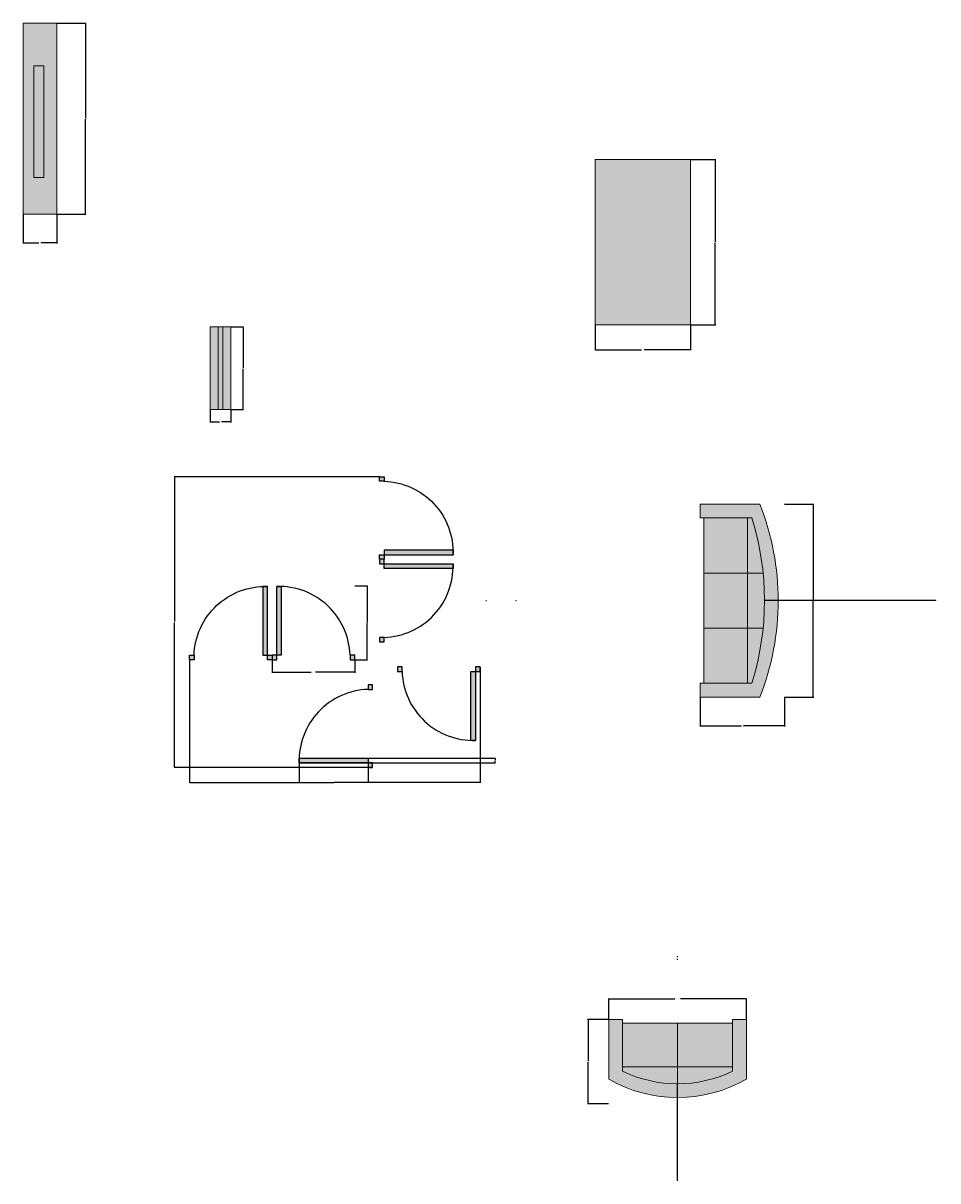
# Model space of a CAD drawing. Units: inches. Extents: x -494 to 1275, y 12 to 1194.
# Tile 5 of 8: x 857 to 1255, y 231 to 735. Entities that reach past the tile are written whole.
import ezdxf

# ---------------------------------------------------------------- set-up
doc = ezdxf.new("R2010")
doc.units = ezdxf.units.IN
doc.header["$MEASUREMENT"] = 0
for name, color, linetype, lineweight in [('A-ANNO-DIMS', 2, 'Continuous', 18), ('A-DOOR', 3, 'Continuous', 25), ('A-DOOR-PATT', 7, 'Continuous', 13), ('A-FURN', 8, 'Continuous', 18), ('A-GLAZ', 4, 'Continuous', 18), ('A-GLAZ-FRAM-PATT', 7, 'Continuous', 13), ('A-GLAZ-GLAS-PATT', 4, 'Continuous', 13)]:
    doc.layers.add(name, color=color, linetype=linetype, lineweight=lineweight)
doc.layers.add('A-FURN-PATT', color=254, linetype='Continuous', lineweight=13, true_color=0xfeeab9)
doc.styles.get("Standard").update_dxf_attribs({"font": 'arial.ttf'})
doc.dimstyles.get("Standard").update_dxf_attribs({"dimtxt": 0.18, "dimasz": 0.18, "dimexe": 0.18, "dimexo": 0.0625, "dimgap": 0.09, "dimtad": 0, "dimtih": 1, "dimtoh": 1, "dimdec": 4, "dimzin": 0, "dimdsep": 46, "dimlunit": 4, "dimtxsty": 'Standard', "dimcen": 0.09, "dimadec": 0, "dimazin": 0, "dimtfac": 1, "dimtdec": 4, "dimtofl": 0, "dimtmove": 0, "dimatfit": 3, "dimfxl": 1, "dimtolj": 1, "dimtzin": 0, "dimarcsym": 0})

# ---------------------------------------------------------------- blocks, each defined once
blk = doc.blocks.new('Sofa - Roundback Loveseat 5 ft.')
for p, q in [((0, -32.44198), (0, -5.99998)), ((-24, -33.99998), (-24, -11.46958)), ((-23.9998, -13.38178), (23.99986, -13.38178)), ((24.00004, -33.99998), (24.00004, -11.46958)), ((-24, -32.44198), (24.00004, -32.44198))]:
    blk.add_line(p, q)
for points in [[(-24, -33.99998), (-30, -33.99998), (-30, -7.99998)], [(30.00004, -7.99998), (30.00004, -33.99998), (24.00004, -33.99998)]]:
    blk.add_lwpolyline(points)
for centre, radius, start, end in [((0, -60.24998), 60.24998, 60.13715, 119.8628), ((0, -61.38438), 55.38444, 64.32083, 115.6792)]:
    blk.add_arc(centre, radius, start, end)
blk = doc.blocks.new('WINDOW-36IN')
for p, q in [((3.5, 36), (3.5, 0)), ((5.5, 36), (5.5, 0))]:
    blk.add_line(p, q)
blk.add_lwpolyline([(0, 36), (9, 36), (9, 0), (0, 0)], close=True)
blk = doc.blocks.new('DOOR-SINGLE-36IN')
blk.add_lwpolyline([(34, 2, 0.414214), (2, 32), (4, 32), (4, 2), (2, 2), (2, 32)], format="xyb")
for points in [[(0, 0), (2, 0), (2, 2), (0, 2)], [(34, 0), (36, 0), (36, 2), (34, 2)]]:
    blk.add_lwpolyline(points, close=True)
blk = doc.blocks.new('SOFA-84IN-PLAN')
h = blk.add_hatch(color=256)
h.dxf.hatch_style = 1
h.paths.add_polyline_path([(20.62, 54), (1.56, 54), (1.56, 30), (20.62, 30)], flags=17)
h.paths.add_polyline_path([(20.62, 78), (1.56, 78), (1.56, 54), (20.62, 54)], flags=17)
h.paths.add_polyline_path([(22.53, 78), (20.62, 78), (20.62, 54), (27.4, 54, 0.050647)], flags=17)
h.paths.add_polyline_path([(27.4, 54), (20.62, 54), (20.62, 30), (27.4, 30, 0.049628)], flags=17)
h.paths.add_polyline_path([(20.62, 30), (1.56, 30), (1.56, 6), (20.62, 6)], flags=17)
h.paths.add_polyline_path([(27.4, 30), (20.62, 30), (20.62, 6), (22.53, 6, 0.050647)], flags=17)
h.paths.add_polyline_path([(26, 84), (0, 84), (0, 78), (22.53, 78, -0.050647), (27.4, 54, -0.100528), (22.53, 6), (20.62, 6), (1.56, 6), (0, 6), (0, 0), (26, 0, 0.190476)])
for p, q in [((0, 78), (22.53, 78)), ((1.56, 78), (1.56, 6)), ((20.62, 78), (20.62, 6)), ((1.56, 54), (27.4, 54)), ((1.56, 30), (27.4, 30)), ((0, 6), (22.53, 6))]:
    blk.add_line(p, q)
for points in [[(0, 78), (0, 84), (26, 84)], [(26, 0), (0, 0), (0, 6)]]:
    blk.add_lwpolyline(points)
for centre, radius, start, end in [((-80.25, 42), 114.25, 338.4314, 21.5686), ((-93.2, 42), 121.2, 342.7203, 17.2797)]:
    blk.add_arc(centre, radius, start, end)
blk = doc.blocks.new('TABLE-RECTANGULAR-72IN')
h = blk.add_hatch(color=256)
h.dxf.hatch_style = 1
h.paths.add_polyline_path([(41.56, 71.99), (0, 71.99), (0, 0), (41.56, 0)])
blk.add_lwpolyline([(0, 0), (41.56, 0), (41.56, 71.99), (0, 71.99)], close=True)
blk = doc.blocks.new('MEDIA-CONSOLE-PLAN')
for p, q in [((4.67, 64.59), (9.03, 64.59)), ((4.67, 16.07), (4.67, 64.59)), ((9.03, 64.59), (9.03, 16.07)), ((9.03, 16.07), (4.67, 16.07))]:
    blk.add_line(p, q)
blk.add_lwpolyline([(0, 83.25), (14.68, 83.25), (14.68, 0), (0, 0)], close=True)
blk = doc.blocks.new('*D18')
at = {"layer": 'A-ANNO-DIMS', "color": 0, "lineweight": -2, "transparency": 16777216}
for p, q in [((965.19, 457.67), (965.19, 452.15)), ((1001.19, 457.67), (1001.19, 452.15)), ((965.37, 452.33), (982.25, 452.33)), ((1001.01, 452.33), (984.12, 452.33))]:
    blk.add_line(p, q, dxfattribs=at)
at = {"layer": 'A-ANNO-DIMS', "color": 0, "transparency": 16777216}
for points in [[(965.37, 452.36), (965.37, 452.3), (965.19, 452.33)], [(1001.01, 452.36), (1001.01, 452.3), (1001.19, 452.33)]]:
    blk.add_solid(points, dxfattribs=at)
at = {"layer": 'Defpoints', "color": 0, "transparency": 16777216}
for p in [(965.19, 457.73), (1001.19, 457.73), (1001.19, 452.33)]:
    blk.add_point(p, dxfattribs=at)
at = {"layer": 'A-ANNO-DIMS', "color": 0, "transparency": 16777216, "insert": (983.19, 452.33), "char_height": 0.18, "attachment_point": 5}
blk.add_mtext('\\A1;DOOR 36 TYP.', dxfattribs=at)
blk = doc.blocks.new('*D19')
at = {"layer": 'A-ANNO-DIMS', "color": 0, "lineweight": -2, "transparency": 16777216}
for p, q in [((1001.25, 490), (1006.77, 490)), ((1006.59, 489.82), (1006.59, 474.05)), ((1006.59, 457.91), (1006.59, 473.68)), ((1001.25, 457.73), (1006.77, 457.73))]:
    blk.add_line(p, q, dxfattribs=at)
at = {"layer": 'A-ANNO-DIMS', "color": 0, "transparency": 16777216}
for points in [[(1006.56, 489.82), (1006.62, 489.82), (1006.59, 490)], [(1006.56, 457.91), (1006.62, 457.91), (1006.59, 457.73)]]:
    blk.add_solid(points, dxfattribs=at)
at = {"layer": 'Defpoints', "color": 0, "transparency": 16777216}
for p in [(1001.19, 490), (1006.59, 490), (1001.19, 457.73)]:
    blk.add_point(p, dxfattribs=at)
at = {"layer": 'A-ANNO-DIMS', "color": 0, "transparency": 16777216, "insert": (1006.59, 473.86), "char_height": 0.18, "attachment_point": 5}
blk.add_mtext('\\A1;32 TYP.', dxfattribs=at)
blk = doc.blocks.new('*D22')
at = {"layer": 'A-ANNO-DIMS', "color": 0, "lineweight": -2, "transparency": 16777216}
for p, q in [((947.28, 602.76), (952.8, 602.76)), ((952.62, 602.58), (952.62, 584.95)), ((952.62, 566.94), (952.62, 584.58)), ((947.28, 566.76), (952.8, 566.76))]:
    blk.add_line(p, q, dxfattribs=at)
at = {"layer": 'A-ANNO-DIMS', "color": 0, "transparency": 16777216}
for points in [[(952.59, 602.58), (952.65, 602.58), (952.62, 602.76)], [(952.59, 566.94), (952.65, 566.94), (952.62, 566.76)]]:
    blk.add_solid(points, dxfattribs=at)
at = {"layer": 'Defpoints', "color": 0, "transparency": 16777216}
for p in [(947.22, 602.76), (952.62, 602.76), (947.22, 566.76)]:
    blk.add_point(p, dxfattribs=at)
at = {"layer": 'A-ANNO-DIMS', "color": 0, "transparency": 16777216, "insert": (952.62, 584.76), "char_height": 0.18, "attachment_point": 5}
blk.add_mtext('\\A1;WINDOW B 36 TYP.', dxfattribs=at)
blk = doc.blocks.new('*D23')
at = {"layer": 'A-ANNO-DIMS', "color": 0, "lineweight": -2, "transparency": 16777216}
for p, q in [((938.22, 566.7), (938.22, 561.18)), ((947.22, 566.7), (947.22, 561.18)), ((938.4, 561.36), (942.26, 561.36)), ((947.04, 561.36), (943.18, 561.36))]:
    blk.add_line(p, q, dxfattribs=at)
at = {"layer": 'A-ANNO-DIMS', "color": 0, "transparency": 16777216}
for points in [[(938.4, 561.39), (938.4, 561.33), (938.22, 561.36)], [(947.04, 561.39), (947.04, 561.33), (947.22, 561.36)]]:
    blk.add_solid(points, dxfattribs=at)
at = {"layer": 'Defpoints', "color": 0, "transparency": 16777216}
for p in [(938.22, 566.76), (947.22, 566.76), (947.22, 561.36)]:
    blk.add_point(p, dxfattribs=at)
at = {"layer": 'A-ANNO-DIMS', "color": 0, "transparency": 16777216, "insert": (942.72, 561.36), "char_height": 0.18, "attachment_point": 5}
blk.add_mtext('\\A1;9 TYP.', dxfattribs=at)
blk = doc.blocks.new('*D28')
at = {"layer": 'A-ANNO-DIMS', "color": 0, "lineweight": -2, "transparency": 16777216}
for p, q in [((1111.85, 301.15), (1111.85, 310.27)), ((1112.03, 310.09), (1140.63, 310.09)), ((1171.67, 310.09), (1143.08, 310.09)), ((1171.85, 301.15), (1171.85, 310.27))]:
    blk.add_line(p, q, dxfattribs=at)
at = {"layer": 'A-ANNO-DIMS', "color": 0, "transparency": 16777216}
for points in [[(1112.03, 310.12), (1112.03, 310.06), (1111.85, 310.09)], [(1171.67, 310.12), (1171.67, 310.06), (1171.85, 310.09)]]:
    blk.add_solid(points, dxfattribs=at)
at = {"layer": 'Defpoints', "color": 0, "transparency": 16777216}
for p in [(1111.85, 310.09), (1111.85, 301.09), (1171.85, 301.09)]:
    blk.add_point(p, dxfattribs=at)
at = {"layer": 'A-ANNO-DIMS', "color": 0, "transparency": 16777216, "insert": (1141.85, 310.09), "char_height": 0.18, "attachment_point": 5}
blk.add_mtext('\\A1;LOVESEAT 60 TYP.', dxfattribs=at)
blk = doc.blocks.new('*D29')
at = {"layer": 'A-ANNO-DIMS', "color": 0, "lineweight": -2, "transparency": 16777216}
for p, q in [((1111.79, 301.09), (1102.67, 301.09)), ((1102.85, 300.91), (1102.85, 282.94)), ((1102.85, 264.6), (1102.85, 282.57)), ((1111.79, 264.42), (1102.67, 264.42))]:
    blk.add_line(p, q, dxfattribs=at)
at = {"layer": 'A-ANNO-DIMS', "color": 0, "transparency": 16777216}
for points in [[(1102.82, 300.91), (1102.88, 300.91), (1102.85, 301.09)], [(1102.82, 264.6), (1102.88, 264.6), (1102.85, 264.42)]]:
    blk.add_solid(points, dxfattribs=at)
at = {"layer": 'Defpoints', "color": 0, "transparency": 16777216}
for p in [(1111.85, 301.09), (1102.85, 264.42), (1111.85, 264.42)]:
    blk.add_point(p, dxfattribs=at)
at = {"layer": 'A-ANNO-DIMS', "color": 0, "transparency": 16777216, "insert": (1102.85, 282.76), "char_height": 0.18, "attachment_point": 5}
blk.add_mtext('\\A1;37 TYP.', dxfattribs=at)
blk = doc.blocks.new('*D32')
at = {"layer": 'A-ANNO-DIMS', "color": 0, "lineweight": -2, "transparency": 16777216}
for p, q in [((1188.46, 525.54), (1201.18, 525.54)), ((1201, 525.36), (1201, 483.73)), ((1201, 441.72), (1201, 483.36)), ((1188.46, 441.54), (1201.18, 441.54))]:
    blk.add_line(p, q, dxfattribs=at)
at = {"layer": 'A-ANNO-DIMS', "color": 0, "transparency": 16777216}
for points in [[(1200.97, 525.36), (1201.03, 525.36), (1201, 525.54)], [(1200.97, 441.72), (1201.03, 441.72), (1201, 441.54)]]:
    blk.add_solid(points, dxfattribs=at)
at = {"layer": 'Defpoints', "color": 0, "transparency": 16777216}
for p in [(1188.4, 525.54), (1201, 525.54), (1188.4, 441.54)]:
    blk.add_point(p, dxfattribs=at)
at = {"layer": 'A-ANNO-DIMS', "color": 0, "transparency": 16777216, "insert": (1201, 483.54), "char_height": 0.18, "attachment_point": 5}
blk.add_mtext('\\A1;SOFA 84 TYP.', dxfattribs=at)
blk = doc.blocks.new('*D33')
at = {"layer": 'A-ANNO-DIMS', "color": 0, "lineweight": -2, "transparency": 16777216}
for p, q in [((1151.73, 441.48), (1151.73, 428.76)), ((1188.4, 441.48), (1188.4, 428.76)), ((1151.91, 428.94), (1169.53, 428.94)), ((1188.22, 428.94), (1170.59, 428.94))]:
    blk.add_line(p, q, dxfattribs=at)
at = {"layer": 'A-ANNO-DIMS', "color": 0, "transparency": 16777216}
for points in [[(1151.91, 428.97), (1151.91, 428.91), (1151.73, 428.94)], [(1188.22, 428.97), (1188.22, 428.91), (1188.4, 428.94)]]:
    blk.add_solid(points, dxfattribs=at)
at = {"layer": 'Defpoints', "color": 0, "transparency": 16777216}
for p in [(1151.73, 441.54), (1188.4, 441.54), (1188.4, 428.94)]:
    blk.add_point(p, dxfattribs=at)
at = {"layer": 'A-ANNO-DIMS', "color": 0, "transparency": 16777216, "insert": (1170.06, 428.94), "char_height": 0.18, "attachment_point": 5}
blk.add_mtext('\\A1;37 TYP.', dxfattribs=at)
blk = doc.blocks.new('*D34')
at = {"layer": 'A-ANNO-DIMS', "color": 0, "lineweight": -2, "transparency": 16777216}
for p, q in [((1147.57, 675.62), (1158.48, 675.62)), ((1158.3, 675.44), (1158.3, 639.81)), ((1158.3, 603.81), (1158.3, 639.44)), ((1147.57, 603.63), (1158.48, 603.63))]:
    blk.add_line(p, q, dxfattribs=at)
at = {"layer": 'A-ANNO-DIMS', "color": 0, "transparency": 16777216}
for points in [[(1158.27, 675.44), (1158.33, 675.44), (1158.3, 675.62)], [(1158.27, 603.81), (1158.33, 603.81), (1158.3, 603.63)]]:
    blk.add_solid(points, dxfattribs=at)
at = {"layer": 'Defpoints', "color": 0, "transparency": 16777216}
for p in [(1147.5, 675.62), (1158.3, 675.62), (1147.5, 603.63)]:
    blk.add_point(p, dxfattribs=at)
at = {"layer": 'A-ANNO-DIMS', "color": 0, "transparency": 16777216, "insert": (1158.3, 639.63), "char_height": 0.18, "attachment_point": 5}
blk.add_mtext('\\A1;TABLE 72 TYP.', dxfattribs=at)
blk = doc.blocks.new('*D35')
at = {"layer": 'A-ANNO-DIMS', "color": 0, "lineweight": -2, "transparency": 16777216}
for p, q in [((1105.94, 603.57), (1105.94, 592.65)), ((1147.5, 603.57), (1147.5, 592.65)), ((1106.12, 592.83), (1126.19, 592.83)), ((1147.32, 592.83), (1127.25, 592.83))]:
    blk.add_line(p, q, dxfattribs=at)
at = {"layer": 'A-ANNO-DIMS', "color": 0, "transparency": 16777216}
for points in [[(1106.12, 592.86), (1106.12, 592.8), (1105.94, 592.83)], [(1147.32, 592.86), (1147.32, 592.8), (1147.5, 592.83)]]:
    blk.add_solid(points, dxfattribs=at)
at = {"layer": 'Defpoints', "color": 0, "transparency": 16777216}
for p in [(1105.94, 603.63), (1147.5, 603.63), (1147.5, 592.83)]:
    blk.add_point(p, dxfattribs=at)
at = {"layer": 'A-ANNO-DIMS', "color": 0, "transparency": 16777216, "insert": (1126.72, 592.83), "char_height": 0.18, "attachment_point": 5}
blk.add_mtext('\\A1;42 TYP.', dxfattribs=at)
blk = doc.blocks.new('*D36')
at = {"layer": 'A-ANNO-DIMS', "color": 0, "lineweight": -2, "transparency": 16777216}
for p, q in [((871.45, 735.08), (884.06, 735.08)), ((883.88, 734.9), (883.88, 693.64)), ((883.88, 652.01), (883.88, 693.27)), ((871.45, 651.83), (884.06, 651.83))]:
    blk.add_line(p, q, dxfattribs=at)
at = {"layer": 'A-ANNO-DIMS', "color": 0, "transparency": 16777216}
for points in [[(883.85, 734.9), (883.91, 734.9), (883.88, 735.08)], [(883.85, 652.01), (883.91, 652.01), (883.88, 651.83)]]:
    blk.add_solid(points, dxfattribs=at)
at = {"layer": 'Defpoints', "color": 0, "transparency": 16777216}
for p in [(871.39, 735.08), (883.88, 735.08), (871.39, 651.83)]:
    blk.add_point(p, dxfattribs=at)
at = {"layer": 'A-ANNO-DIMS', "color": 0, "transparency": 16777216, "insert": (883.88, 693.45), "char_height": 0.18, "attachment_point": 5}
blk.add_mtext('\\A1;CONSOLE 83 TYP.', dxfattribs=at)
blk = doc.blocks.new('*D37')
at = {"layer": 'A-ANNO-DIMS', "color": 0, "lineweight": -2, "transparency": 16777216}
for p, q in [((856.71, 651.77), (856.71, 639.16)), ((871.39, 651.77), (871.39, 639.16)), ((856.89, 639.34), (863.53, 639.34)), ((871.21, 639.34), (864.57, 639.34))]:
    blk.add_line(p, q, dxfattribs=at)
at = {"layer": 'A-ANNO-DIMS', "color": 0, "transparency": 16777216}
for points in [[(856.89, 639.37), (856.89, 639.31), (856.71, 639.34)], [(871.21, 639.37), (871.21, 639.31), (871.39, 639.34)]]:
    blk.add_solid(points, dxfattribs=at)
at = {"layer": 'Defpoints', "color": 0, "transparency": 16777216}
for p in [(856.71, 651.83), (871.39, 651.83), (871.39, 639.34)]:
    blk.add_point(p, dxfattribs=at)
at = {"layer": 'A-ANNO-DIMS', "color": 0, "transparency": 16777216, "insert": (864.05, 639.34), "char_height": 0.18, "attachment_point": 5}
blk.add_mtext('\\A1;15 TYP.', dxfattribs=at)
blk = doc.blocks.new('*D76')
at = {"layer": 'A-ANNO-DIMS', "color": 0, "lineweight": -2, "transparency": 16777216}
for p, q in [((929.19, 457.67), (929.19, 404.15)), ((1055.84, 454.62), (1055.84, 404.15)), ((929.37, 404.33), (992.06, 404.33)), ((1055.66, 404.33), (992.97, 404.33))]:
    blk.add_line(p, q, dxfattribs=at)
at = {"layer": 'A-ANNO-DIMS', "color": 0, "transparency": 16777216}
for points in [[(929.37, 404.36), (929.37, 404.3), (929.19, 404.33)], [(1055.66, 404.36), (1055.66, 404.3), (1055.84, 404.33)]]:
    blk.add_solid(points, dxfattribs=at)
at = {"layer": 'Defpoints', "color": 0, "transparency": 16777216}
for p in [(929.19, 457.73), (1055.84, 454.69), (1055.84, 404.33)]:
    blk.add_point(p, dxfattribs=at)
at = {"layer": 'A-ANNO-DIMS', "color": 0, "transparency": 16777216, "insert": (992.51, 404.33), "char_height": 0.18, "attachment_point": 5}
blk.add_mtext('\\A1;126.66', dxfattribs=at)
blk = doc.blocks.new('*D77')
at = {"layer": 'A-ANNO-DIMS', "color": 0, "lineweight": -2, "transparency": 16777216}
for p, q in [((1011.97, 537.54), (922.46, 537.54)), ((922.64, 537.36), (922.64, 474.39)), ((922.64, 411.06), (922.64, 474.03)), ((1008.93, 410.88), (922.46, 410.88))]:
    blk.add_line(p, q, dxfattribs=at)
at = {"layer": 'A-ANNO-DIMS', "color": 0, "transparency": 16777216}
for points in [[(922.61, 537.36), (922.67, 537.36), (922.64, 537.54)], [(922.61, 411.06), (922.67, 411.06), (922.64, 410.88)]]:
    blk.add_solid(points, dxfattribs=at)
at = {"layer": 'Defpoints', "color": 0, "transparency": 16777216}
for p in [(922.64, 537.54), (1012.04, 537.54), (1008.99, 410.88)]:
    blk.add_point(p, dxfattribs=at)
at = {"layer": 'A-ANNO-DIMS', "color": 0, "transparency": 16777216, "insert": (922.64, 474.21), "char_height": 0.18, "attachment_point": 5}
blk.add_mtext('\\A1;126.66', dxfattribs=at)
blk = doc.blocks.new('*D95')
at = {"layer": 'A-ANNO-DIMS', "color": 0, "lineweight": -2, "transparency": 16777216}
for p, q in [((976.99, 412.82), (976.99, 404.15)), ((1006.99, 412.82), (1006.99, 404.15)), ((977.17, 404.33), (991.77, 404.33)), ((1006.81, 404.33), (992.21, 404.33))]:
    blk.add_line(p, q, dxfattribs=at)
at = {"layer": 'A-ANNO-DIMS', "color": 0, "transparency": 16777216}
for points in [[(977.17, 404.36), (977.17, 404.3), (976.99, 404.33)], [(1006.81, 404.36), (1006.81, 404.3), (1006.99, 404.33)]]:
    blk.add_solid(points, dxfattribs=at)
at = {"layer": 'Defpoints', "color": 0, "transparency": 16777216}
for p in [(976.99, 412.88), (1006.99, 412.88), (1006.99, 404.33)]:
    blk.add_point(p, dxfattribs=at)
at = {"layer": 'A-ANNO-DIMS', "color": 0, "transparency": 16777216, "insert": (991.99, 404.33), "char_height": 0.18, "attachment_point": 5}
blk.add_mtext('\\A1;30', dxfattribs=at)
blk = doc.blocks.new('*D96')
at = {"layer": 'A-ANNO-DIMS', "color": 0, "lineweight": -2, "transparency": 16777216}
for p, q in [((977.05, 414.88), (1062.57, 414.88)), ((1062.39, 414.7), (1062.39, 414.06)), ((1062.39, 413.06), (1062.39, 413.7)), ((977.05, 412.88), (1062.57, 412.88))]:
    blk.add_line(p, q, dxfattribs=at)
at = {"layer": 'A-ANNO-DIMS', "color": 0, "transparency": 16777216}
for points in [[(1062.36, 414.7), (1062.42, 414.7), (1062.39, 414.88)], [(1062.36, 413.06), (1062.42, 413.06), (1062.39, 412.88)]]:
    blk.add_solid(points, dxfattribs=at)
at = {"layer": 'Defpoints', "color": 0, "transparency": 16777216}
for p in [(976.99, 414.88), (1062.39, 414.88), (976.99, 412.88)]:
    blk.add_point(p, dxfattribs=at)
at = {"layer": 'A-ANNO-DIMS', "color": 0, "transparency": 16777216, "insert": (1062.39, 413.88), "char_height": 0.18, "attachment_point": 5}
blk.add_mtext('\\A1;2', dxfattribs=at)
blk = doc.blocks.new('*D109')
at = {"layer": 'A-ANNO-DIMS', "color": 0, "lineweight": -2, "transparency": 16777216}
for p, q in [((1071.39, 483.54), (1071.57, 483.54)), ((1071.48, 483.45), (1071.48, 483.63)), ((1254.28, 483.54), (1185.91, 483.54))]:
    blk.add_line(p, q, dxfattribs=at)
at = {"layer": 'A-ANNO-DIMS', "color": 0, "transparency": 16777216}
blk.add_solid([(1185.91, 483.57), (1185.91, 483.51), (1185.73, 483.54)], dxfattribs=at)
at = {"layer": 'Defpoints', "color": 0, "transparency": 16777216}
for p in [(1071.48, 483.54), (1185.73, 483.54)]:
    blk.add_point(p, dxfattribs=at)
at = {"layer": 'A-ANNO-DIMS', "color": 0, "transparency": 16777216, "insert": (1254.83, 483.54), "char_height": 0.18, "attachment_point": 5}
blk.add_mtext('\\A1;R114.25', dxfattribs=at)
blk = doc.blocks.new('*D110')
at = {"layer": 'A-ANNO-DIMS', "color": 0, "lineweight": -2, "transparency": 16777216}
for p, q in [((1058.44, 483.54), (1058.62, 483.54)), ((1058.53, 483.45), (1058.53, 483.63)), ((1252.45, 483.54), (1179.91, 483.54))]:
    blk.add_line(p, q, dxfattribs=at)
at = {"layer": 'A-ANNO-DIMS', "color": 0, "transparency": 16777216}
blk.add_solid([(1179.91, 483.57), (1179.91, 483.51), (1179.73, 483.54)], dxfattribs=at)
at = {"layer": 'Defpoints', "color": 0, "transparency": 16777216}
for p in [(1058.53, 483.54), (1179.73, 483.54)]:
    blk.add_point(p, dxfattribs=at)
at = {"layer": 'A-ANNO-DIMS', "color": 0, "transparency": 16777216, "insert": (1252.93, 483.54), "char_height": 0.18, "attachment_point": 5}
blk.add_mtext('\\A1;R121.2', dxfattribs=at)
blk = doc.blocks.new('*D111')
at = {"layer": 'A-ANNO-DIMS', "color": 0, "lineweight": -2, "transparency": 16777216}
for p, q in [((1141.76, 327.34), (1141.94, 327.34)), ((1141.85, 327.25), (1141.85, 327.43)), ((1141.85, 230.94), (1141.85, 266.91)), ((1142.04, 230.94), (1141.85, 230.94))]:
    blk.add_line(p, q, dxfattribs=at)
at = {"layer": 'A-ANNO-DIMS', "color": 0, "transparency": 16777216}
blk.add_solid([(1141.89, 266.91), (1141.83, 266.91), (1141.85, 267.09)], dxfattribs=at)
at = {"layer": 'Defpoints', "color": 0, "transparency": 16777216}
for p in [(1141.85, 327.34), (1141.85, 267.09)]:
    blk.add_point(p, dxfattribs=at)
at = {"layer": 'A-ANNO-DIMS', "color": 0, "transparency": 16777216, "insert": (1142.52, 230.94), "char_height": 0.18, "attachment_point": 5}
blk.add_mtext('\\A1;R60.25', dxfattribs=at)
blk = doc.blocks.new('*D112')
at = {"layer": 'A-ANNO-DIMS', "color": 0, "lineweight": -2, "transparency": 16777216}
for p, q in [((1141.76, 328.47), (1141.94, 328.47)), ((1141.85, 328.38), (1141.85, 328.56)), ((1141.85, 239.86), (1141.85, 272.91)), ((1142.04, 239.86), (1141.85, 239.86))]:
    blk.add_line(p, q, dxfattribs=at)
at = {"layer": 'A-ANNO-DIMS', "color": 0, "transparency": 16777216}
blk.add_solid([(1141.89, 272.91), (1141.83, 272.91), (1141.85, 273.09)], dxfattribs=at)
at = {"layer": 'Defpoints', "color": 0, "transparency": 16777216}
for p in [(1141.85, 328.47), (1141.85, 273.09)]:
    blk.add_point(p, dxfattribs=at)
at = {"layer": 'A-ANNO-DIMS', "color": 0, "transparency": 16777216, "insert": (1142.52, 239.86), "char_height": 0.18, "attachment_point": 5}
blk.add_mtext('\\A1;R55.38', dxfattribs=at)

msp = doc.modelspace()

# ---------------------------------------------------------------- hatches: boundary and pattern name
at = {"layer": 'A-DOOR-PATT'}
h = msp.add_hatch(color=256, dxfattribs=at)
h.dxf.hatch_style = 1
h.paths.add_polyline_path([(1044.0365, 503.5367), (1044.0365, 505.5367), (1014.0365, 505.5367), (1014.0365, 503.5367)])
h.paths.add_polyline_path([(1012.0365, 501.5367), (1014.0365, 501.5367), (1014.0365, 503.5367), (1012.0365, 503.5367)])
h.paths.add_polyline_path([(1014.0365, 535.5367), (1014.0365, 537.5367), (1012.0365, 537.5367), (1012.0365, 535.5367)])
h = msp.add_hatch(color=256, dxfattribs=at)
h.dxf.hatch_style = 1
h.paths.add_polyline_path([(1014.0365, 499.5367), (1014.0365, 497.5367), (1044.0365, 497.5367), (1044.0365, 499.5367)])
h.paths.add_polyline_path([(1012.0365, 499.5367), (1014.0365, 499.5367), (1014.0365, 501.5367), (1012.0365, 501.5367)])
h.paths.add_polyline_path([(1012.0365, 467.5367), (1012.0365, 465.5367), (1014.0365, 465.5367), (1014.0365, 467.5367)])
h = msp.add_hatch(color=256, dxfattribs=at)
h.dxf.hatch_style = 1
h.paths.add_polyline_path([(963.1857, 489.7319), (961.1857, 489.7319), (961.1857, 459.7319), (963.1857, 459.7319)])
h.paths.add_polyline_path([(965.1857, 457.7319), (965.1857, 459.7319), (963.1857, 459.7319), (963.1857, 457.7319)])
h.paths.add_polyline_path([(931.1857, 459.7319), (929.1857, 459.7319), (929.1857, 457.7319), (931.1857, 457.7319)])
h = msp.add_hatch(color=256, dxfattribs=at)
h.dxf.hatch_style = 1
h.paths.add_polyline_path([(967.1857, 459.7319), (969.1857, 459.7319), (969.1857, 489.7319), (967.1857, 489.7319)])
h.paths.add_polyline_path([(967.1857, 457.7319), (967.1857, 459.7319), (965.1857, 459.7319), (965.1857, 457.7319)])
h.paths.add_polyline_path([(999.1857, 457.7319), (1001.1857, 457.7319), (1001.1857, 459.7319), (999.1857, 459.7319)])
h = msp.add_hatch(color=256, dxfattribs=at)
h.dxf.hatch_style = 1
h.paths.add_polyline_path([(1053.8413, 452.6859), (1051.8413, 452.6859), (1051.8413, 422.6859), (1053.8413, 422.6859)])
h.paths.add_polyline_path([(1053.8413, 454.6859), (1053.8413, 452.6859), (1055.8413, 452.6859), (1055.8413, 454.6859)])
h.paths.add_polyline_path([(1021.8413, 454.6859), (1019.8413, 454.6859), (1019.8413, 452.6859), (1021.8413, 452.6859)])
h = msp.add_hatch(color=256, dxfattribs=at)
h.dxf.hatch_style = 1
h.paths.add_polyline_path([(1006.9905, 412.8811), (1006.9905, 414.8811), (976.9905, 414.8811), (976.9905, 412.8811)])
h.paths.add_polyline_path([(1008.9905, 412.8811), (1006.9905, 412.8811), (1006.9905, 410.8811), (1008.9905, 410.8811)])
h.paths.add_polyline_path([(1008.9905, 444.8811), (1008.9905, 446.8811), (1006.9905, 446.8811), (1006.9905, 444.8811)])
at = {"layer": 'A-FURN-PATT'}
h = msp.add_hatch(color=256, dxfattribs=at)
h.dxf.hatch_style = 1
h.paths.add_polyline_path([(856.7136, 651.8301), (871.3923, 651.8301), (871.3923, 735.0769), (856.7136, 735.0769)])
h.paths.add_polyline_path([(861.3852, 667.9018), (861.3852, 716.4203), (865.7447, 716.4203), (865.7447, 667.9018)], flags=16)
h = msp.add_hatch(color=256, dxfattribs=at)
h.dxf.hatch_style = 1
h.paths.add_polyline_path([(865.7447, 716.4203), (861.3852, 716.4203), (861.3852, 667.9018), (865.7447, 667.9018)])
h = msp.add_hatch(color=256, dxfattribs=at)
h.dxf.hatch_style = 1
h.paths.add_polyline_path([(1165.8549, 299.5316), (1141.8549, 299.5316), (1141.8549, 280.4714), (1165.8549, 280.4714)], flags=17)
h.paths.add_polyline_path([(1117.8549, 299.5316), (1117.8549, 280.4714), (1141.8549, 280.4714), (1141.8549, 299.5316)], flags=17)
h.paths.add_polyline_path([(1141.8549, 273.0896), (1141.8549, 280.4714), (1117.8549, 280.4714), (1117.8549, 278.5598, 0.11251889)], flags=16)
h.paths.add_polyline_path([(1165.8549, 278.5597), (1165.8549, 280.4714), (1141.8549, 280.4714), (1141.8549, 273.0896, 0.11251869)], flags=17)
h.paths.add_polyline_path([(1117.8549, 278.5598), (1117.8549, 301.0896), (1111.8549, 301.0896), (1111.8549, 275.0897, 0.26666697), (1171.8549, 275.0896), (1171.8549, 301.0896), (1165.8549, 301.0896), (1165.8549, 278.5597, -0.22792319)])
at = {"layer": 'A-GLAZ-FRAM-PATT'}
h = msp.add_hatch(color=256, dxfattribs=at)
h.dxf.hatch_style = 1
h.paths.add_polyline_path([(941.7213, 602.762), (938.2213, 602.762), (938.2213, 566.762), (941.7213, 566.762)])
h.paths.add_polyline_path([(943.7213, 566.762), (947.2213, 566.762), (947.2213, 602.762), (943.7213, 602.762)])
at = {"layer": 'A-GLAZ-GLAS-PATT'}
h = msp.add_hatch(color=256, dxfattribs=at)
h.dxf.hatch_style = 1
h.paths.add_polyline_path([(941.7213, 566.762), (943.7213, 566.762), (943.7213, 602.762), (941.7213, 602.762)])

# ---------------------------------------------------------------- linework, layer by layer
at = {"layer": 'A-DOOR'}
for p, q in [((1012.0365, 535.5367), (1012.0365, 537.5367)), ((1012.0365, 501.5367), (1012.0365, 503.5367)), ((1012.0365, 501.5367), (1012.0365, 499.5367)), ((1012.0365, 467.5367), (1012.0365, 465.5367)), ((931.1857, 457.7319), (929.1857, 457.7319)), ((965.1857, 457.7319), (963.1857, 457.7319)), ((965.1857, 457.7319), (967.1857, 457.7319)), ((999.1857, 457.7319), (1001.1857, 457.7319)), ((1021.8413, 454.6859), (1019.8413, 454.6859)), ((1055.8413, 454.6859), (1053.8413, 454.6859)), ((1008.9905, 444.8811), (1008.9905, 446.8811)), ((1008.9905, 410.8811), (1008.9905, 412.8811))]:
    msp.add_line(p, q, dxfattribs=at)

# ---------------------------------------------------------------- block references
at = {"layer": 'A-DOOR', "extrusion": (0, 0, -1), "zscale": -1, "rotation": 89.99999999999955}
msp.add_blockref('DOOR-SINGLE-36IN', (-1012.0366, 501.537), dxfattribs=at)
at = {"layer": 'A-DOOR'}
for p, rotation in [((1012.0366, 501.5364), 269.9999999999996), ((1055.841, 454.6858), 180), ((1008.9904, 410.8814), 90.0000000000003)]:
    msp.add_blockref('DOOR-SINGLE-36IN', p, dxfattribs=dict(at, rotation=rotation))
at = {"layer": 'A-DOOR', "extrusion": (0, 0, -1), "zscale": -1}
msp.add_blockref('DOOR-SINGLE-36IN', (-965.1854, 457.732), dxfattribs=at)
at = {"layer": 'A-DOOR'}
msp.add_blockref('DOOR-SINGLE-36IN', (965.186, 457.732), dxfattribs=at)
at = {"layer": 'A-FURN'}
for name, p in [('MEDIA-CONSOLE-PLAN', (856.714, 651.83)), ('TABLE-RECTANGULAR-72IN', (1105.941, 603.63)), ('SOFA-84IN-PLAN', (1151.73, 441.543))]:
    msp.add_blockref(name, p, dxfattribs=at)
at = {"layer": 'A-FURN', "rotation": 180}
msp.add_blockref('Sofa - Roundback Loveseat 5 ft.', (1141.8549, 267.0896), dxfattribs=at)
at = {"layer": 'A-GLAZ'}
msp.add_blockref('WINDOW-36IN', (938.221, 566.762), dxfattribs=at)

# ---------------------------------------------------------------- dimensions: what is measured, and where the dimension line sits
at = {"layer": 'A-ANNO-DIMS'}
for base, p1, p2, angle, text, picture, middle in [((883.8793, 735.0769), (871.3923, 651.8301), (871.3923, 735.0769), 90, 'CONSOLE <> TYP.', '*D36', (883.8793, 693.4535)), ((1158.3033, 675.6205), (1147.5047, 603.6298), (1147.5047, 675.6205), 90, 'TABLE <> TYP.', '*D34', (1158.3033, 639.6252)), ((952.6213, 602.762), (947.2213, 566.762), (947.2213, 602.762), 90, 'WINDOW B <> TYP.', '*D22', (952.6213, 584.762)), ((1200.9963, 525.5428), (1188.3963, 441.5428), (1188.3963, 525.5428), 90, 'SOFA <> TYP.', '*D32', (1200.9963, 483.5428)), ((1006.5857, 489.9972), (1001.1857, 457.7319), (1001.1857, 489.9972), 90, '<> TYP.', '*D19', (1006.5857, 473.8645)), ((1111.8549, 310.0896), (1171.8549, 301.0896), (1111.8549, 301.0896), 180, 'LOVESEAT <> TYP.', '*D28', (1141.8549, 310.0896)), ((1102.8549, 264.423), (1111.8549, 301.0896), (1111.8549, 264.423), 270, '<> TYP.', '*D29', (1102.8549, 282.7563))]:
    dim = msp.add_linear_dim(base=base, p1=p1, p2=p2, angle=angle, text=text, dimstyle='Standard', override={"dimdec": 0, "dimlfac": 1, "dimrnd": 0, "dimzin": 0, "dimdsep": 46, "dimlunit": 2}, dxfattribs=at)
    dim.commit()
    dim.dimension.update_dxf_attribs({"geometry": picture, "text_midpoint": middle})
for base, p1, p2, text, picture, middle in [((871.3923, 639.343), (856.7136, 651.8301), (871.3923, 651.8301), '<> TYP.', '*D37', (864.053, 639.343)), ((1147.5047, 592.8312), (1105.9408, 603.6298), (1147.5047, 603.6298), '<> TYP.', '*D35', (1126.7227, 592.8312)), ((947.2213, 561.362), (938.2213, 566.762), (947.2213, 566.762), '<> TYP.', '*D23', (942.7213, 561.362)), ((1001.1857, 452.3319), (965.1857, 457.7319), (1001.1857, 457.7319), 'DOOR <> TYP.', '*D18', (983.1857, 452.3319)), ((1188.3963, 428.9428), (1151.7296, 441.5428), (1188.3963, 441.5428), '<> TYP.', '*D33', (1170.063, 428.9428))]:
    dim = msp.add_linear_dim(base=base, p1=p1, p2=p2, text=text, dimstyle='Standard', override={"dimdec": 0, "dimlfac": 1, "dimrnd": 0, "dimzin": 0, "dimdsep": 46, "dimlunit": 2}, dxfattribs=at)
    dim.commit()
    dim.dimension.update_dxf_attribs({"geometry": picture, "text_midpoint": middle})
for base, p1, p2, override, picture, middle in [((922.6357, 537.5367), (1008.9905, 410.8811), (1012.0365, 537.5367), {"dimdec": 2, "dimlfac": 1, "dimrnd": 0, "dimzin": 0, "dimdsep": 46, "dimlunit": 2}, '*D77', (922.6357, 474.2089)), ((1062.3913, 414.8811), (976.9905, 412.8811), (976.9905, 414.8811), {"dimdec": 0, "dimlfac": 1, "dimrnd": 0, "dimzin": 0, "dimdsep": 46, "dimlunit": 2}, '*D96', (1062.3913, 413.8811))]:
    dim = msp.add_linear_dim(base=base, p1=p1, p2=p2, angle=90, dimstyle='Standard', override=override, dxfattribs=at)
    dim.commit()
    dim.dimension.update_dxf_attribs({"geometry": picture, "text_midpoint": middle})
for center, mpoint, override, picture, middle in [((1058.5328, 483.5428), (1179.7296, 483.543), {"dimdec": 1, "dimlfac": 1, "dimrnd": 0, "dimzin": 0, "dimdsep": 46, "dimlunit": 2}, '*D110', (1252.4477, 483.5431)), ((1071.4796, 483.5428), (1185.7296, 483.543), {"dimdec": 2, "dimlfac": 1, "dimrnd": 0, "dimzin": 0, "dimdsep": 46, "dimlunit": 2}, '*D109', (1254.2796, 483.5431)), ((1141.8549, 328.474), (1141.855, 273.0896), {"dimdec": 2, "dimlfac": 1, "dimrnd": 0, "dimzin": 0, "dimdsep": 46, "dimlunit": 2}, '*D112', (1142.5151, 239.8589)), ((1141.8549, 327.3396), (1141.855, 267.0896), {"dimdec": 2, "dimlfac": 1, "dimrnd": 0, "dimzin": 0, "dimdsep": 46, "dimlunit": 2}, '*D111', (1142.5156, 230.9397))]:
    dim = msp.add_radius_dim(center=center, mpoint=mpoint, dimstyle='Standard', override=override, dxfattribs=at)
    dim.commit()
    dim.dimension.update_dxf_attribs({"geometry": picture, "text_midpoint": middle, "dimtype": 164})
for base, p1, p2, override, picture, middle in [((1055.8413, 404.3311), (929.1857, 457.7319), (1055.8413, 454.6859), {"dimdec": 2, "dimlfac": 1, "dimrnd": 0, "dimzin": 0, "dimdsep": 46, "dimlunit": 2}, '*D76', (992.5135, 404.3311)), ((1006.9905, 404.3311), (976.9905, 412.8811), (1006.9905, 412.8811), {"dimdec": 0, "dimlfac": 1, "dimrnd": 0, "dimzin": 0, "dimdsep": 46, "dimlunit": 2}, '*D95', (991.9905, 404.3311))]:
    dim = msp.add_linear_dim(base=base, p1=p1, p2=p2, dimstyle='Standard', override=override, dxfattribs=at)
    dim.commit()
    dim.dimension.update_dxf_attribs({"geometry": picture, "text_midpoint": middle})

doc.saveas('drawing.dxf')
